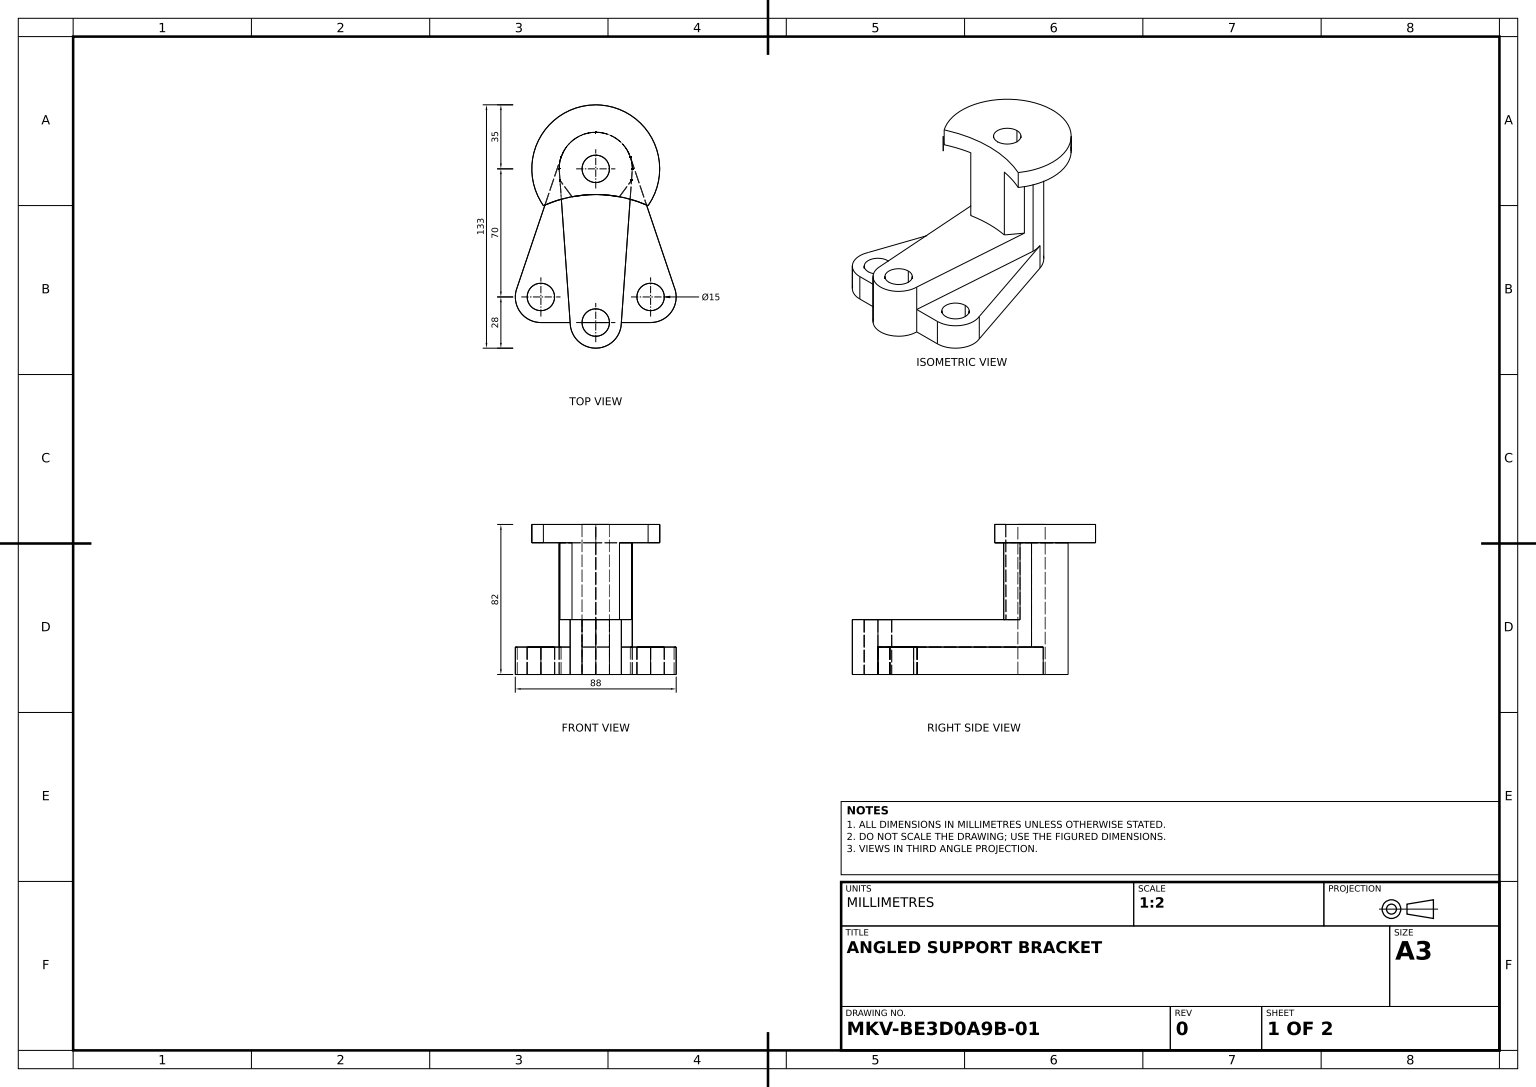
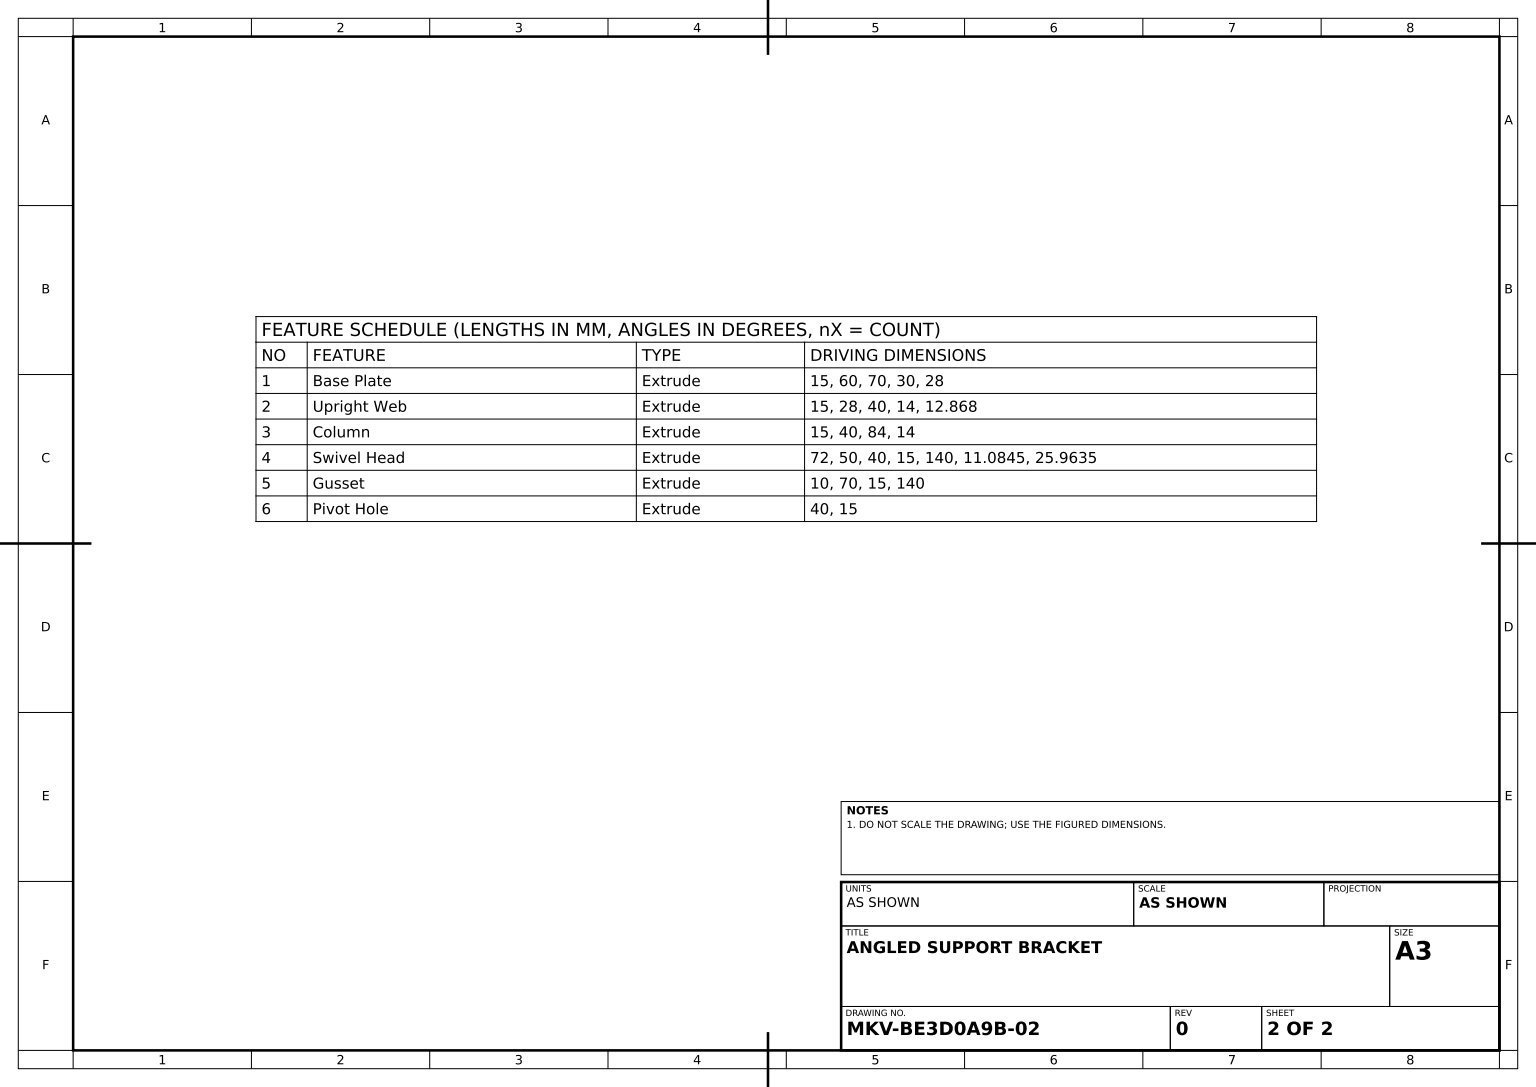
SolidWorks part; units mm, degrees
material "Plain Carbon Steel"
ref_plane "Front Plane" through (0, 0, 0) normal (0, 0, 1) x (1, 0, 0)
ref_plane "Top Plane" through (0, 0, 0) normal (0, 1, 0) x (1, 0, 0)
ref_plane "Right Plane" through (0, 0, 0) normal (1, 0, 0) x (0, 0, -1)
sketch "Base Plate Sketch" plane through (0, 0, 0) normal (0, 1, 0) x (1, 0, 0)
  line L0 (17.132, 75.5149) -> (-12.868, 5.5149)
  line L1 (0, -14) -> (60, -14)
  line L2 (42.868, 75.5149) -> (72.868, 5.5149)
  circle A0 centre (0, 0) radius 7.5
  circle A1 centre (60, 0) radius 7.5
  circle A2 centre (30, 70) radius 7.5
  arc A3 (42.868, 75.5149) -> (17.132, 75.5149) centre (30, 70) ccw
  arc A4 (-12.868, 5.5149) -> (0, -14) centre (0, 0) ccw
  arc A5 (60, -14) -> (72.868, 5.5149) centre (60, 0) ccw
  dimension "D1" = 15
  dimension "D2" = 15
  dimension "D3" = 15
  dimension "D7" = 28
  dimension "D8" = 28
  dimension "D9" = 28
  dimension "D4" = 60
  dimension "D5" = 70
  dimension "D6" = 30
extrude "Base Plate" add sketch "Base Plate Sketch" along normal blind 15
sketch "Upright Web Sketch" plane through (0, 0, 0) normal (0, -1, 0) x (1, 0, 0)
  line L3 (-12.868, -5.5149) -> (11.0498, -76.3946)
  line L4 (72.868, -5.5149) -> (48.9502, -76.3946)
  line L5 (0, 14) -> (16, 14)
  line L6 (44, 14) -> (60, 14)
  arc A0 (44, 14) -> (16, 14) centre (30, 14) ccw
  circle A1 centre (30, 14) radius 7.5
  arc A2 (11.0498, -76.3946) -> (48.9502, -76.3946) centre (30, -70) ccw
  arc A3 (-12.868, -5.5149) -> (0, 14) centre (0, 0) cw
  arc A4 (60, 14) -> (72.868, -5.5149) centre (60, 0) cw
  circle A5 centre (0, 0) radius 7.5
  circle A6 centre (60, 0) radius 7.5
  dimension "D1" = 15
  dimension "D2" = 28
  dimension "D4" = 40
  dimension "D5" = 15
  dimension "D6" = 15
  dimension "D3" = 14
  dimension "D7" = 12.868
extrude "Upright Web" add sketch "Upright Web Sketch" against normal blind 15
sketch "Column Sketch" plane through (0, 15, 0) normal (0, 1, 0) x (1, 0, 0)
  line L0 (10, 70) -> (16, -14)
  line L1 (44, -14) -> (50, 70)
  arc A0 (49.797, 67.1574) -> (10.203, 67.1574) centre (30, 70) ccw
  arc A1 (16, -14) -> (44, -14) centre (30, -14) ccw construction
  arc A2 (16, -14) -> (44, -14) centre (30, -14) ccw
  arc A3 (22.5, -14) -> (37.5, -14) centre (30, -14) ccw
  circle A4 centre (30, -14) radius 7.5
  arc M5 (16, -14) -> (44, -14) centre (30, -14) ccw
  arc M9 (48.9502, 76.3946) -> (11.0498, 76.3946) centre (30, 70) ccw
  arc M10 (37.5, -14) -> (22.5, -14) centre (30, -14) cw
  dimension "D1" = 40
  dimension "D3" = 14
  dimension "D4" = 15
  dimension "D2" = 84
extrude "Column" add sketch "Column Sketch" along normal blind 15 contours L1 A0 L0 A4 M9 M5 M10
ref_plane "Swivel Head Plane" through (0, 72, 0) normal (0, 1, 0) x (1, 0, 0)
sketch "Swivel Head Sketch" plane through (0, 72, 0) normal (0, 1, 0) x (1, 0, 0)
  line L0 (22.5, -14) -> (37.5, -14) construction
  line L2 (42.9817, 54.7857) -> (49.551, 63.7138)
  line L3 (44, -14) -> (50, 70) construction
  line L4 (17.0183, 54.7857) -> (10.449, 63.7138)
  line L5 (10, 70) -> (16, -14) construction
  line L6 (49.551, 63.7138) -> (50, 70)
  line L7 (10.449, 63.7138) -> (10, 70)
  circle A0 centre (30, 70) radius 7.5
  arc A1 (49.797, 67.1574) -> (10.203, 67.1574) centre (30, 70) ccw
  arc A2 (42.9817, 54.7857) -> (17.0183, 54.7857) centre (30, -14) ccw
  dimension "D1" = 40
  dimension "D2" = 15
  dimension "D3" = 140
  dimension "D4" = 11.0845
  dimension "D5" = 25.9635
extrude "Swivel Head" add sketch "Swivel Head Sketch" against normal blind 50 contours A2 L2 L6 A1 L7 L4 A0
sketch "Gusset Sketch" plane through (0, 72, 0) normal (0, 1, 0) x (1, 0, 0)
  line L0 (22.5, -14) -> (37.5, -14) construction
  arc A0 (58.6354, 49.875) -> (1.3646, 49.875) centre (30, 70) ccw
  circle A1 centre (30, 70) radius 7.5
  arc A2 (58.6354, 49.875) -> (1.3646, 49.875) centre (30, -14) ccw
  dimension "D1" = 70
  dimension "D2" = 15
  dimension "D3" = 140
extrude "Gusset" add sketch "Gusset Sketch" along normal blind 10
sketch "Pivot Hole Sketch" plane through (0, 30, 0) normal (0, 1, 0) x (1, 0, 0)
  circle A0 centre (30, 70) radius 7.5
  dimension "D1" = 15
extrude "Pivot Hole" cut sketch "Pivot Hole Sketch" against normal blind 40
